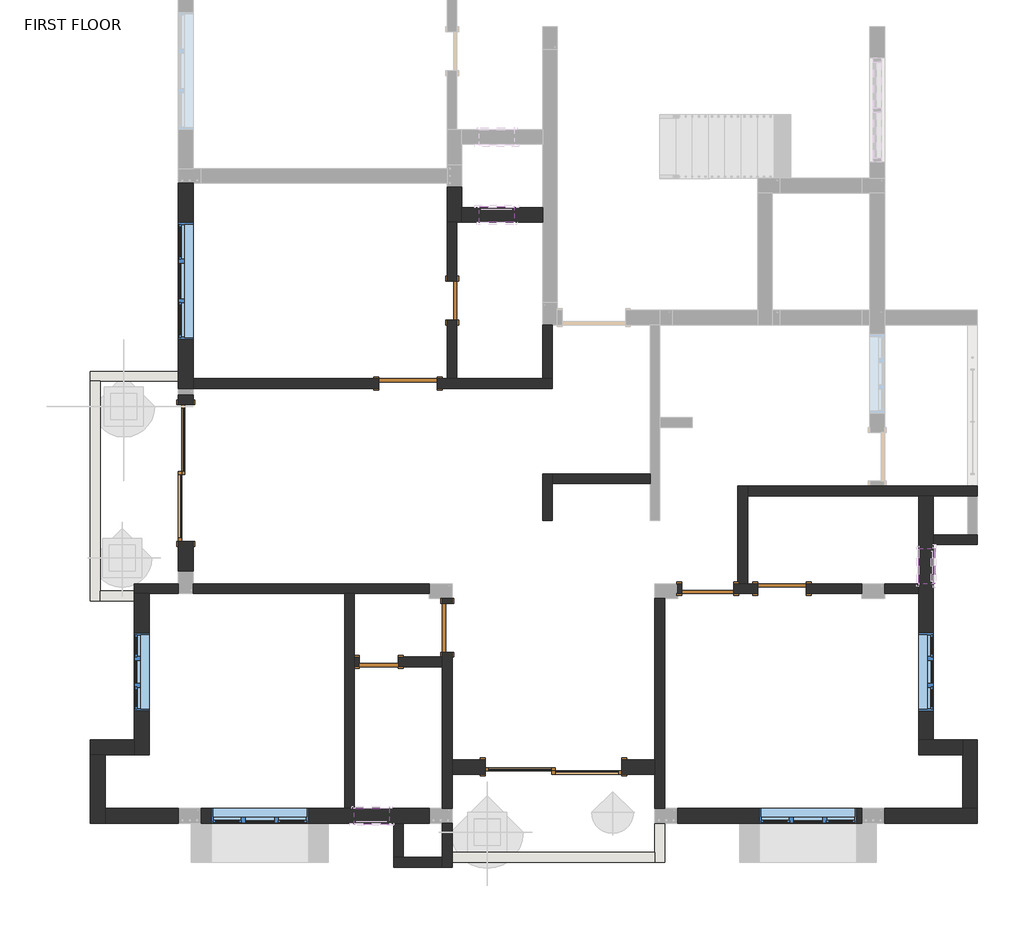
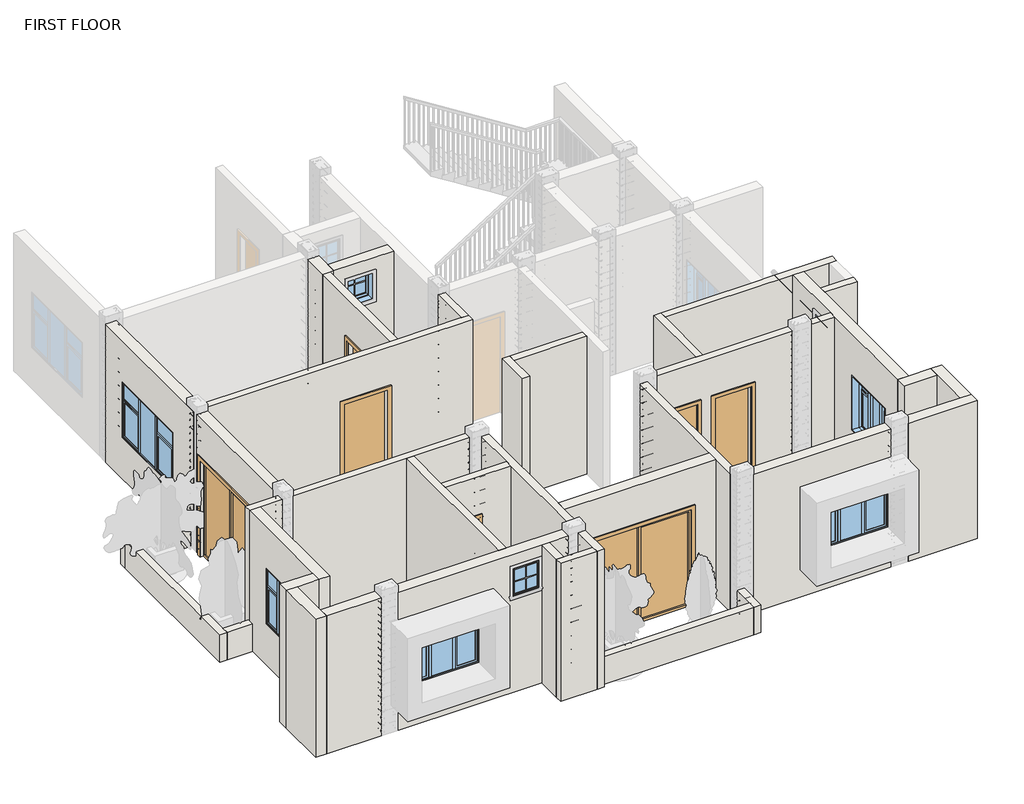
# One storey, part 1 of 10: 39 walls, 8 doors, 8 windows.
"""IFC4 building model written with IfcOpenShell, lengths in millimetres."""

from ifc_helpers import new_model, si_unit, frame, origin, place, context, project, spatial, polyline, outline, extrude, faceted_brep, transform, mapped, element, save
from components import door_double_sliding_7_x7_ddbaaa7c, door_e2b13fe9, door_377e7377, single_flush_2_x7_9ea4ff49, single_flush_3_x7_16372e1c, window_casement_triple_side_transom_4_x4_2_fd24aed3, window_casement_triple_side_transom_5_x4_f59ddf0b, window_casement_triple_side_transom_6_x4_596ba82f, window_6ec6991e

model = new_model("IFC4")

# Units and contexts
model_context = context("Model", 3, world=origin())
ifc_project = project(units=[si_unit("LENGTHUNIT", "METRE", prefix="MILLI")], contexts=[model_context])

# Site, building, storey
site = spatial("IfcSite", under=ifc_project)
building = spatial("IfcBuilding", under=site)
storey = spatial("IfcBuildingStorey", under=building, Name="FIRST FLOOR", Elevation=3200.4)

# Doors
placement = place(None, origin())
door_double_sliding_7_x7_shape = door_double_sliding_7_x7_ddbaaa7c(model_context)
element("IfcDoor", 1, ObjectType="Door-Double-Sliding : 7'X7'", at=placement, inside=storey, context=model_context, shape_type="MappedRepresentation", body=[
    mapped(door_double_sliding_7_x7_shape, transform((-403.8333787, -9045.640066, 3200.4), x_axis=(-1.0, 0.0, 0.0), y_axis=(0.0, -1.0, 0.0), z_axis=(0.0, 0.0, 1.0))),
])
element("IfcDoor", 2, ObjectType="Door-Double-Sliding : 7'X7'", at=placement, inside=storey, context=model_context, shape_type="MappedRepresentation", body=[
    mapped(door_double_sliding_7_x7_shape, transform((-6010.8833787, -4587.940066, 3200.4), x_axis=(0.0, 1.0, 0.0), y_axis=(-1.0, 0.0, 0.0), z_axis=(0.0, 0.0, 1.0))),
])
door_shape = door_e2b13fe9(model_context)
element("IfcDoor", 3, ObjectType="Single-Flush : 2'6\"X7'", at=placement, inside=storey, context=model_context, shape_type="MappedRepresentation", body=[
    mapped(door_shape, transform((-2061.1833787, -7000.940066, 3200.4), x_axis=(0.0, -1.0, 0.0), y_axis=(1.0, 0.0, 0.0), z_axis=(0.0, 0.0, 1.0))),
])
element("IfcDoor", 4, ObjectType="Single-Flush : 2'6\"X7'", at=placement, inside=storey, context=model_context, shape_type="MappedRepresentation", body=[
    mapped(door_shape, transform((3158.5166213, -6391.340066, 3200.4), x_axis=(-1.0, 0.0, 0.0), y_axis=(0.0, -1.0, 0.0), z_axis=(0.0, 0.0, 1.0))),
])
door_2_shape = door_377e7377(model_context)
element("IfcDoor", 5, ObjectType="Single-Flush : 2'8\"X7'", at=placement, inside=storey, context=model_context, shape_type="MappedRepresentation", body=[
    mapped(door_2_shape, transform((2002.8166213, -6391.340066, 3200.4), x_axis=(-1.0, 0.0, 0.0), y_axis=(0.0, -1.0, 0.0), z_axis=(0.0, 0.0, 1.0))),
])
single_flush_2_x7_shape = single_flush_2_x7_9ea4ff49(model_context)
element("IfcDoor", 6, ObjectType="Single-Flush : 2'X7'", at=placement, inside=storey, context=model_context, shape_type="MappedRepresentation", body=[
    mapped(single_flush_2_x7_shape, transform((-3127.9833787, -7534.340066, 3200.4), x_axis=(-1.0, 0.0, 0.0), y_axis=(0.0, -1.0, 0.0), z_axis=(0.0, 0.0, 1.0))),
])
element("IfcDoor", 7, ObjectType="Single-Flush : 2'X7'", at=placement, inside=storey, context=model_context, shape_type="MappedRepresentation", body=[
    mapped(single_flush_2_x7_shape, transform((-1984.9833787, -1895.540066, 3200.4), x_axis=(0.0, -1.0, 0.0), y_axis=(1.0, 0.0, 0.0), z_axis=(0.0, 0.0, 1.0))),
])
single_flush_3_x7_shape = single_flush_3_x7_16372e1c(model_context)
element("IfcDoor", 8, ObjectType="Single-Flush : 3'X7'", at=placement, inside=storey, context=model_context, shape_type="MappedRepresentation", body=[
    mapped(single_flush_3_x7_shape, transform((-2670.7833787, -3190.940066, 3200.4), x_axis=(1.0, 0.0, 0.0), y_axis=(0.0, 1.0, 0.0), z_axis=(0.0, 0.0, 1.0))),
])

# Walls
element("IfcWall", 9, ObjectType="6\"", at=placement, inside=storey, context=model_context, shape_type="SweptSolid", body=[
    extrude(outline(polyline([(-2200.340066, 5334.0), (-2200.340066, 3200.4), (-3114.740066, 3200.4), (-3114.740066, 6248.4), (-676.340066, 6248.4), (-676.340066, 3200.4), (-1590.740066, 3200.4), (-1590.740066, 5334.0), (-2200.340066, 5334.0)])), frame((-2061.1833787, 0.0, 0.0), z_axis=(1.0, 0.0, 0.0), x_axis=(0.0, 1.0, 0.0)), (0.0, 0.0, 1.0), 152.4),
])
element("IfcWall", 10, ObjectType="6\"", at=placement, inside=storey, context=model_context, shape_type="Brep", body=[
    faceted_brep([(-2213.5833787, -3267.140066, 5334.0), (-2213.5833787, -3267.140066, 3200.4), (-422.8833787, -3267.140066, 3200.4), (-422.8833787, -3267.140066, 6248.4), (-6023.5833787, -3267.140066, 6248.4), (-6023.5833787, -3267.140066, 3810.0), (-6023.5833787, -3267.140066, 3200.4), (-3127.9833787, -3267.140066, 3200.4), (-3127.9833787, -3267.140066, 5334.0), (-422.8833787, -3114.740066, 3200.4), (-575.2833787, -3114.740066, 3200.4), (-1908.7833787, -3114.740066, 3200.4), (-2061.1833787, -3114.740066, 3200.4), (-2213.5833787, -3114.740066, 3200.4), (-2213.5833787, -3114.740066, 5334.0), (-3127.9833787, -3114.740066, 5334.0), (-3127.9833787, -3114.740066, 3200.4), (-6023.5833787, -3114.740066, 3200.4), (-6023.5833787, -3114.740066, 6248.4), (-2061.1833787, -3114.740066, 6248.4), (-1908.7833787, -3114.740066, 6248.4), (-575.2833787, -3114.740066, 6248.4), (-422.8833787, -3114.740066, 6248.4), (-6023.5833787, -3152.840066, 3200.4)], [[[0, 1, 2, 3, 4, 5, 6, 7, 8]], [[9, 10, 11, 12, 13, 14, 15, 16, 17, 18, 19, 20, 21, 22]], [[7, 6, 23, 17, 16]], [[2, 1, 13, 12, 11, 10, 9]], [[4, 3, 22, 21, 20, 19, 18]], [[3, 2, 9, 22]], [[14, 13, 1, 0]], [[15, 14, 0, 8]], [[16, 15, 8, 7]], [[6, 5, 4, 18, 17, 23]]]),
])
element("IfcWall", 11, ObjectType="6\"", at=placement, inside=storey, context=model_context, shape_type="SweptSolid", body=[
    extrude(outline(polyline([(-422.8833787, -2276.540066), (-422.8833787, -3114.740066), (-575.2833787, -3114.740066), (-575.2833787, -2276.540066), (-422.8833787, -2276.540066)])), frame((0.0, 0.0, 3200.4), z_axis=(0.0, 0.0, 1.0), x_axis=(1.0, 0.0, 0.0)), (0.0, 0.0, 1.0), 3048.0),
])
element("IfcWall", 12, ObjectType="6\"", at=placement, inside=storey, context=model_context, shape_type="Brep", body=[
    faceted_brep([(-6937.9833787, -6467.540066, 6248.4), (-6937.9833787, -6467.540066, 3200.4), (-6709.3833787, -6467.540066, 3200.4), (-6252.1833787, -6467.540066, 3200.4), (-6252.1833787, -6467.540066, 6248.4), (-6709.3833787, -6467.540066, 6248.4), (-6937.9833787, -6315.140066, 3200.4), (-6937.9833787, -6315.140066, 6248.4), (-6252.1833787, -6315.140066, 6248.4), (-6252.1833787, -6315.140066, 3200.4), (-6937.9833787, -6429.440066, 3200.4)], [[[0, 1, 2, 3, 4, 5]], [[6, 7, 8, 9]], [[3, 2, 1, 10, 6, 9]], [[4, 3, 9, 8]], [[0, 5, 4, 8, 7]], [[0, 7, 6, 10, 1]]]),
])
element("IfcWall", 13, ObjectType="6\"", at=placement, inside=storey, context=model_context, shape_type="Brep", body=[
    faceted_brep([(-6023.5833787, -6467.540066, 3200.4), (-3661.3833787, -6467.540066, 3200.4), (-3508.9833787, -6467.540066, 3200.4), (-2340.5833787, -6467.540066, 3200.4), (-2340.5833787, -6467.540066, 6248.4), (-3508.9833787, -6467.540066, 6248.4), (-3661.3833787, -6467.540066, 6248.4), (-6023.5833787, -6467.540066, 6248.4), (-6023.5833787, -6315.140066, 3200.4), (-6023.5833787, -6315.140066, 6248.4), (-2340.5833787, -6315.140066, 6248.4), (-2340.5833787, -6315.140066, 3200.4)], [[[0, 1, 2, 3, 4, 5, 6, 7]], [[8, 9, 10, 11]], [[3, 2, 1, 0, 8, 11]], [[4, 3, 11, 10]], [[7, 6, 5, 4, 10, 9]], [[0, 7, 9, 8]]]),
])
element("IfcWall", 14, ObjectType="6\"", at=placement, inside=storey, context=model_context, shape_type="Brep", body=[
    faceted_brep([(-3508.9833787, -9820.340066, 3200.4), (-3508.9833787, -7610.540066, 3200.4), (-3508.9833787, -7458.140066, 3200.4), (-3508.9833787, -6467.540066, 3200.4), (-3508.9833787, -6467.540066, 6248.4), (-3508.9833787, -7458.140066, 6248.4), (-3508.9833787, -7610.540066, 6248.4), (-3508.9833787, -9820.340066, 6248.4), (-3508.9833787, -9820.340066, 5943.6), (-3508.9833787, -9820.340066, 5334.0), (-3661.3833787, -9820.340066, 3200.4), (-3661.3833787, -9820.340066, 6248.4), (-3661.3833787, -6467.540066, 6248.4), (-3661.3833787, -6467.540066, 3200.4)], [[[0, 1, 2, 3, 4, 5, 6, 7, 8, 9]], [[10, 11, 12, 13]], [[3, 2, 1, 0, 10, 13]], [[7, 6, 5, 4, 12, 11]], [[0, 9, 8, 7, 11, 10]], [[4, 3, 13, 12]]]),
])
element("IfcWall", 15, ObjectType="6\"", at=placement, inside=storey, context=model_context, shape_type="Brep", body=[
    faceted_brep([(-1984.9833787, -9820.340066, 3200.4), (-1984.9833787, -9286.940066, 3200.4), (-1984.9833787, -9058.340066, 3200.4), (-1984.9833787, -7381.940066, 3200.4), (-1984.9833787, -7381.940066, 5334.0), (-1984.9833787, -6619.940066, 5334.0), (-1984.9833787, -6619.940066, 3200.4), (-1984.9833787, -6543.740066, 3200.4), (-1984.9833787, -6543.740066, 6248.4), (-1984.9833787, -9058.340066, 6248.4), (-1984.9833787, -9286.940066, 6248.4), (-1984.9833787, -9820.340066, 6248.4), (-2137.3833787, -7381.940066, 5334.0), (-2137.3833787, -7381.940066, 3200.4), (-2137.3833787, -7458.140066, 3200.4), (-2137.3833787, -7610.540066, 3200.4), (-2137.3833787, -9820.340066, 3200.4), (-2137.3833787, -9820.340066, 6248.4), (-2137.3833787, -7610.540066, 6248.4), (-2137.3833787, -7458.140066, 6248.4), (-2137.3833787, -6543.740066, 6248.4), (-2137.3833787, -6543.740066, 3200.4), (-2137.3833787, -6619.940066, 3200.4), (-2137.3833787, -6619.940066, 5334.0)], [[[0, 1, 2, 3, 4, 5, 6, 7, 8, 9, 10, 11]], [[12, 13, 14, 15, 16, 17, 18, 19, 20, 21, 22, 23]], [[22, 21, 7, 6]], [[16, 15, 14, 13, 3, 2, 1, 0]], [[8, 7, 21, 20]], [[11, 10, 9, 8, 20, 19, 18, 17]], [[0, 11, 17, 16]], [[4, 3, 13, 12]], [[5, 4, 12, 23]], [[6, 5, 23, 22]]]),
])
element("IfcWall", 16, ObjectType="6\"", at=placement, inside=storey, context=model_context, shape_type="SweptSolid", body=[
    extrude(outline(polyline([(3200.4, -3508.9833787), (3200.4, -3432.7833787), (5334.0, -3432.7833787), (5334.0, -2823.1833787), (3200.4, -2823.1833787), (3200.4, -2137.3833787), (6248.4, -2137.3833787), (6248.4, -3508.9833787), (3200.4, -3508.9833787)])), frame((0.0, -7610.540066, 0.0), z_axis=(0.0, 1.0, 0.0), x_axis=(0.0, 0.0, 1.0)), (0.0, 0.0, 1.0), 152.4),
])
element("IfcWall", 17, ObjectType="6\"", at=placement, inside=storey, context=model_context, shape_type="Brep", body=[
    faceted_brep([(-2137.3833787, -10048.940066, 3200.4), (-2137.3833787, -10582.340066, 3200.4), (-2137.3833787, -10734.740066, 3200.4), (-2137.3833787, -10734.740066, 6248.4), (-2137.3833787, -10582.340066, 6248.4), (-2137.3833787, -10048.940066, 6248.4), (-1984.9833787, -10048.940066, 3200.4), (-1984.9833787, -10048.940066, 6248.4), (-1984.9833787, -10734.740066, 6248.4), (-1984.9833787, -10734.740066, 3200.4), (-1984.9833787, -10658.540066, 3200.4), (-1984.9833787, -10506.140066, 3200.4)], [[[0, 1, 2, 3, 4, 5]], [[6, 7, 8, 9, 10, 11]], [[2, 1, 0, 6, 11, 10, 9]], [[5, 4, 3, 8, 7]], [[0, 5, 7, 6]], [[2, 9, 8, 3]]]),
])
element("IfcWall", 18, ObjectType="6\"", at=placement, inside=storey, context=model_context, shape_type="Brep", body=[
    faceted_brep([(-2137.3833787, -10582.340066, 6248.4), (-2137.3833787, -10582.340066, 3200.4), (-2746.3100526, -10582.340066, 3200.4), (-2898.7100526, -10582.340066, 3200.4), (-2898.7100526, -10582.340066, 6248.4), (-2746.3100526, -10582.340066, 6248.4), (-2137.3833787, -10734.740066, 3200.4), (-2137.3833787, -10734.740066, 6248.4), (-2898.7100526, -10734.740066, 6248.4), (-2898.7100526, -10734.740066, 3200.4)], [[[0, 1, 2, 3, 4, 5]], [[6, 7, 8, 9]], [[3, 2, 1, 6, 9]], [[0, 5, 4, 8, 7]], [[4, 3, 9, 8]], [[0, 7, 6, 1]]]),
])
element("IfcWall", 19, ObjectType="6\"", at=placement, inside=storey, context=model_context, shape_type="SweptSolid", body=[
    extrude(outline(polyline([(-2746.3100526, -10048.940066), (-2746.3100526, -10582.340066), (-2898.7100526, -10582.340066), (-2898.7100526, -10048.940066), (-2746.3100526, -10048.940066)])), frame((0.0, 0.0, 3200.4), z_axis=(0.0, 0.0, 1.0), x_axis=(1.0, 0.0, 0.0)), (0.0, 0.0, 1.0), 3048.0),
])
element("IfcWall", 20, ObjectType="6\"", at=placement, inside=storey, context=model_context, shape_type="Brep", body=[
    faceted_brep([(1177.3166213, -10048.940066, 3200.4), (1177.3166213, -10506.140066, 3200.4), (1177.3166213, -10658.540066, 3200.4), (1177.3166213, -10658.540066, 3810.0), (1177.3166213, -10506.140066, 3810.0), (1177.3166213, -10048.940066, 3810.0), (1329.7166213, -10048.940066, 3200.4), (1329.7166213, -10048.940066, 3810.0), (1329.7166213, -10658.540066, 3810.0), (1329.7166213, -10658.540066, 3200.4)], [[[0, 1, 2, 3, 4, 5]], [[6, 7, 8, 9]], [[2, 1, 0, 6, 9]], [[5, 4, 3, 8, 7]], [[0, 5, 7, 6]], [[3, 2, 9, 8]]]),
])
element("IfcWall", 21, ObjectType="6\"", at=placement, inside=storey, context=model_context, shape_type="SweptSolid", body=[
    extrude(outline(polyline([(-1984.9833787, -10506.140066), (1177.3166213, -10506.140066), (1177.3166213, -10658.540066), (-1984.9833787, -10658.540066), (-1984.9833787, -10506.140066)])), frame((0.0, 0.0, 3200.4), z_axis=(0.0, 0.0, 1.0), x_axis=(1.0, 0.0, 0.0)), (0.0, 0.0, 1.0), 609.6),
])
element("IfcWall", 22, ObjectType="6\"", at=placement, inside=storey, context=model_context, shape_type="Brep", body=[
    faceted_brep([(1329.7166213, -9820.340066, 3200.4), (1329.7166213, -6543.740066, 3200.4), (1329.7166213, -6543.740066, 6248.4), (1329.7166213, -9820.340066, 6248.4), (1177.3166213, -9820.340066, 3200.4), (1177.3166213, -9820.340066, 6248.4), (1177.3166213, -9286.940066, 6248.4), (1177.3166213, -9058.340066, 6248.4), (1177.3166213, -6543.740066, 6248.4), (1177.3166213, -6543.740066, 3200.4), (1177.3166213, -9058.340066, 3200.4), (1177.3166213, -9286.940066, 3200.4)], [[[0, 1, 2, 3]], [[4, 5, 6, 7, 8, 9, 10, 11]], [[1, 0, 4, 11, 10, 9]], [[2, 1, 9, 8]], [[3, 2, 8, 7, 6, 5]], [[0, 3, 5, 4]]]),
])
element("IfcWall", 23, ObjectType="6\"", at=placement, inside=storey, context=model_context, shape_type="Brep", body=[
    faceted_brep([(2409.2166213, -6467.540066, 3200.4), (2777.5166213, -6467.540066, 3200.4), (2777.5166213, -6467.540066, 5334.0), (3539.5166213, -6467.540066, 5334.0), (3539.5166213, -6467.540066, 3200.4), (4403.1166213, -6467.540066, 3200.4), (4403.1166213, -6467.540066, 6248.4), (1532.9166213, -6467.540066, 6248.4), (1532.9166213, -6467.540066, 3200.4), (1596.4166213, -6467.540066, 3200.4), (1596.4166213, -6467.540066, 5334.0), (2409.2166213, -6467.540066, 5334.0), (2777.5166213, -6315.140066, 5334.0), (2777.5166213, -6315.140066, 3200.4), (2625.1166213, -6315.140066, 3200.4), (2472.7166213, -6315.140066, 3200.4), (2409.2166213, -6315.140066, 3200.4), (2409.2166213, -6315.140066, 5334.0), (1596.4166213, -6315.140066, 5334.0), (1596.4166213, -6315.140066, 3200.4), (1532.9166213, -6315.140066, 3200.4), (1532.9166213, -6315.140066, 6248.4), (2472.7166213, -6315.140066, 6248.4), (2625.1166213, -6315.140066, 6248.4), (4403.1166213, -6315.140066, 6248.4), (4403.1166213, -6315.140066, 3200.4), (3539.5166213, -6315.140066, 3200.4), (3539.5166213, -6315.140066, 5334.0)], [[[0, 1, 2, 3, 4, 5, 6, 7, 8, 9, 10, 11]], [[12, 13, 14, 15, 16, 17, 18, 19, 20, 21, 22, 23, 24, 25, 26, 27]], [[20, 19, 9, 8]], [[26, 25, 5, 4]], [[16, 15, 14, 13, 1, 0]], [[6, 5, 25, 24]], [[7, 6, 24, 23, 22, 21]], [[8, 7, 21, 20]], [[10, 9, 19, 18]], [[11, 10, 18, 17]], [[0, 11, 17, 16]], [[2, 1, 13, 12]], [[3, 2, 12, 27]], [[4, 3, 27, 26]]]),
])
element("IfcWall", 24, ObjectType="6\"", at=placement, inside=storey, context=model_context, shape_type="SweptSolid", body=[
    extrude(outline(polyline([(5292.1166213, -6467.540066), (4758.7166213, -6467.540066), (4758.7166213, -6315.140066), (5292.1166213, -6315.140066), (5292.1166213, -6467.540066)])), frame((0.0, 0.0, 3200.4), z_axis=(0.0, 0.0, 1.0), x_axis=(1.0, 0.0, 0.0)), (0.0, 0.0, 1.0), 3048.0),
])
element("IfcWall", 25, ObjectType="6\"", at=placement, inside=storey, context=model_context, shape_type="Brep", body=[
    faceted_brep([(2625.1166213, -6315.140066, 3200.4), (2625.1166213, -4943.540066, 3200.4), (2625.1166213, -4791.140066, 3200.4), (2625.1166213, -4791.140066, 6248.4), (2625.1166213, -4943.540066, 6248.4), (2625.1166213, -6315.140066, 6248.4), (2472.7166213, -6315.140066, 3200.4), (2472.7166213, -6315.140066, 6248.4), (2472.7166213, -4791.140066, 6248.4), (2472.7166213, -4791.140066, 3200.4)], [[[0, 1, 2, 3, 4, 5]], [[6, 7, 8, 9]], [[2, 1, 0, 6, 9]], [[5, 4, 3, 8, 7]], [[0, 5, 7, 6]], [[3, 2, 9, 8]]]),
])
element("IfcWall", 26, ObjectType="6\"", at=placement, inside=storey, context=model_context, shape_type="Brep", body=[
    faceted_brep([(2625.1166213, -4943.540066, 3200.4), (5292.1166213, -4943.540066, 3200.4), (5520.7166213, -4943.540066, 3200.4), (6054.1166213, -4943.540066, 3200.4), (6054.1166213, -4943.540066, 3810.0), (6206.5166213, -4943.540066, 3810.0), (6206.5166213, -4943.540066, 6248.4), (6054.1166213, -4943.540066, 6248.4), (5520.7166213, -4943.540066, 6248.4), (5292.1166213, -4943.540066, 6248.4), (2625.1166213, -4943.540066, 6248.4), (2625.1166213, -4791.140066, 3200.4), (2625.1166213, -4791.140066, 6248.4), (4530.1166213, -4791.140066, 6248.4), (4758.7166213, -4791.140066, 6248.4), (6206.5166213, -4791.140066, 6248.4), (6206.5166213, -4791.140066, 3810.0), (6054.1166213, -4791.140066, 3810.0), (6054.1166213, -4791.140066, 3200.4), (4758.7166213, -4791.140066, 3200.4), (4530.1166213, -4791.140066, 3200.4)], [[[0, 1, 2, 3, 4, 5, 6, 7, 8, 9, 10]], [[11, 12, 13, 14, 15, 16, 17, 18, 19, 20]], [[3, 2, 1, 0, 11, 20, 19, 18]], [[10, 9, 8, 7, 6, 15, 14, 13, 12]], [[0, 10, 12, 11]], [[16, 5, 4, 17]], [[4, 3, 18, 17]], [[6, 5, 16, 15]]]),
])
element("IfcWall", 27, ObjectType="6\"", at=placement, inside=storey, context=model_context, shape_type="Brep", body=[
    faceted_brep([(-422.8833787, -5324.540066, 3200.4), (-422.8833787, -4753.040066, 3200.4), (-422.8833787, -4600.640066, 3200.4), (-422.8833787, -4600.640066, 6248.4), (-422.8833787, -4753.040066, 6248.4), (-422.8833787, -5324.540066, 6248.4), (-575.2833787, -5324.540066, 3200.4), (-575.2833787, -5324.540066, 6248.4), (-575.2833787, -4600.640066, 6248.4), (-575.2833787, -4600.640066, 3200.4)], [[[0, 1, 2, 3, 4, 5]], [[6, 7, 8, 9]], [[2, 1, 0, 6, 9]], [[5, 4, 3, 8, 7]], [[0, 5, 7, 6]], [[3, 2, 9, 8]]]),
])
element("IfcWall", 28, ObjectType="6\"", at=placement, inside=storey, context=model_context, shape_type="SweptSolid", body=[
    extrude(outline(polyline([(1101.1166213, -4753.040066), (-422.8833787, -4753.040066), (-422.8833787, -4600.640066), (1101.1166213, -4600.640066), (1101.1166213, -4753.040066)])), frame((0.0, 0.0, 3200.4), z_axis=(0.0, 0.0, 1.0), x_axis=(1.0, 0.0, 0.0)), (0.0, 0.0, 1.0), 3048.0),
])
element("IfcWall", 29, ObjectType="6\"", at=placement, inside=storey, context=model_context, shape_type="Brep", body=[
    faceted_brep([(6206.5166213, -5552.4667399, 3200.4), (6054.1166213, -5552.4667399, 3200.4), (5520.7166213, -5552.4667399, 3200.4), (5520.7166213, -5552.4667399, 6248.4), (6054.1166213, -5552.4667399, 6248.4), (6206.5166213, -5552.4667399, 6248.4), (6206.5166213, -5704.8667399, 3200.4), (6206.5166213, -5704.8667399, 6248.4), (5520.7166213, -5704.8667399, 6248.4), (5520.7166213, -5704.8667399, 3200.4)], [[[0, 1, 2, 3, 4, 5]], [[6, 7, 8, 9]], [[2, 1, 0, 6, 9]], [[5, 4, 3, 8, 7]], [[3, 2, 9, 8]], [[0, 5, 7, 6]]]),
])
element("IfcWall", 30, ObjectType="6\"", at=placement, inside=storey, context=model_context, shape_type="Brep", body=[
    faceted_brep([(-6252.1833787, -3000.440066, 3200.4), (-7623.7833787, -3000.440066, 3200.4), (-7623.7833787, -3000.440066, 3810.0), (-6252.1833787, -3000.440066, 3810.0), (-6252.1833787, -3152.840066, 3200.4), (-6252.1833787, -3152.840066, 3810.0), (-7471.3833787, -3152.840066, 3810.0), (-7623.7833787, -3152.840066, 3810.0), (-7623.7833787, -3152.840066, 3200.4), (-7471.3833787, -3152.840066, 3200.4)], [[[0, 1, 2, 3]], [[4, 5, 6, 7, 8, 9]], [[1, 0, 4, 9, 8]], [[3, 2, 7, 6, 5]], [[0, 3, 5, 4]], [[2, 1, 8, 7]]]),
])
element("IfcWall", 31, ObjectType="6\"", at=placement, inside=storey, context=model_context, shape_type="Brep", body=[
    faceted_brep([(-7623.7833787, -3152.840066, 3200.4), (-7623.7833787, -6581.840066, 3200.4), (-7623.7833787, -6581.840066, 3810.0), (-7623.7833787, -3152.840066, 3810.0), (-7471.3833787, -3152.840066, 3200.4), (-7471.3833787, -3152.840066, 3810.0), (-7471.3833787, -6429.440066, 3810.0), (-7471.3833787, -6581.840066, 3810.0), (-7471.3833787, -6581.840066, 3200.4), (-7471.3833787, -6429.440066, 3200.4)], [[[0, 1, 2, 3]], [[4, 5, 6, 7, 8, 9]], [[1, 0, 4, 9, 8]], [[3, 2, 7, 6, 5]], [[0, 3, 5, 4]], [[2, 1, 8, 7]]]),
])
element("IfcWall", 32, ObjectType="6\"", at=placement, inside=storey, context=model_context, shape_type="Brep", body=[
    faceted_brep([(-7471.3833787, -6581.840066, 3200.4), (-6937.9833787, -6581.840066, 3200.4), (-6937.9833787, -6581.840066, 3810.0), (-7471.3833787, -6581.840066, 3810.0), (-7471.3833787, -6429.440066, 3200.4), (-7471.3833787, -6429.440066, 3810.0), (-6937.9833787, -6429.440066, 3810.0), (-6937.9833787, -6429.440066, 3200.4), (-6937.9833787, -6467.540066, 3200.4)], [[[0, 1, 2, 3]], [[4, 5, 6, 7]], [[1, 0, 4, 7, 8]], [[3, 2, 6, 5]], [[0, 3, 5, 4]], [[2, 1, 8, 7, 6]]]),
])
element("IfcWall", 33, ObjectType="9\"", at=placement, inside=storey, context=model_context, shape_type="Brep", body=[
    faceted_brep([(-6252.1833787, -66.740066, 3200.4), (-6252.1833787, -3000.440066, 3200.4), (-6252.1833787, -3152.840066, 3200.4), (-6252.1833787, -3152.840066, 3810.0), (-6252.1833787, -3267.140066, 3810.0), (-6252.1833787, -3267.140066, 6248.4), (-6252.1833787, -66.740066, 6248.4), (-6252.1833787, -676.340066, 5334.0), (-6252.1833787, -2505.140066, 5334.0), (-6252.1833787, -2505.140066, 4114.8), (-6252.1833787, -676.340066, 4114.8), (-6023.5833787, -66.740066, 3200.4), (-6023.5833787, -66.740066, 6248.4), (-6023.5833787, -3114.740066, 6248.4), (-6023.5833787, -3267.140066, 6248.4), (-6023.5833787, -3267.140066, 3810.0), (-6023.5833787, -3152.840066, 3810.0), (-6023.5833787, -3152.840066, 3200.4), (-6023.5833787, -3114.740066, 3200.4), (-6023.5833787, -676.340066, 5334.0), (-6023.5833787, -676.340066, 4114.8), (-6023.5833787, -2505.140066, 4114.8), (-6023.5833787, -2505.140066, 5334.0)], [[[0, 1, 2, 3, 4, 5, 6], [7, 8, 9, 10]], [[11, 12, 13, 14, 15, 16, 17, 18], [19, 20, 21, 22]], [[2, 1, 0, 11, 18, 17]], [[6, 5, 14, 13, 12]], [[0, 6, 12, 11]], [[20, 19, 7, 10]], [[21, 20, 10, 9]], [[22, 21, 9, 8]], [[19, 22, 8, 7]], [[15, 4, 3, 16]], [[3, 2, 17, 16]], [[5, 4, 15, 14]]]),
])
element("IfcWall", 34, ObjectType="9\"", at=placement, inside=storey, context=model_context, shape_type="SweptSolid", body=[
    extrude(outline(polyline([(-3368.740066, 3200.4), (-3521.140066, 3200.4), (-3521.140066, 5334.0), (-5654.740066, 5334.0), (-5654.740066, 3200.4), (-6111.940066, 3200.4), (-6111.940066, 6248.4), (-3368.740066, 6248.4), (-3368.740066, 3200.4)])), frame((-6252.1833787, 0.0, 0.0), z_axis=(1.0, 0.0, 0.0), x_axis=(0.0, 1.0, 0.0)), (0.0, 0.0, 1.0), 228.6),
])
element("IfcWall", 35, ObjectType="9\"", at=placement, inside=storey, context=model_context, shape_type="Brep", body=[
    faceted_brep([(-6937.9833787, -6467.540066, 3200.4), (-6937.9833787, -6581.840066, 3200.4), (-6937.9833787, -8753.540066, 3200.4), (-6937.9833787, -8982.140066, 3200.4), (-6937.9833787, -8982.140066, 6248.4), (-6937.9833787, -8753.540066, 6248.4), (-6937.9833787, -6467.540066, 6248.4), (-6937.9833787, -7079.7633095, 5334.0), (-6937.9833787, -8298.9633095, 5334.0), (-6937.9833787, -8298.9633095, 4114.8), (-6937.9833787, -7079.7633095, 4114.8), (-6709.3833787, -6467.540066, 3200.4), (-6709.3833787, -6467.540066, 6248.4), (-6709.3833787, -8982.140066, 6248.4), (-6709.3833787, -8982.140066, 3200.4), (-6709.3833787, -7079.7633095, 5334.0), (-6709.3833787, -7079.7633095, 4114.8), (-6709.3833787, -8298.9633095, 4114.8), (-6709.3833787, -8298.9633095, 5334.0)], [[[0, 1, 2, 3, 4, 5, 6], [7, 8, 9, 10]], [[11, 12, 13, 14], [15, 16, 17, 18]], [[3, 2, 1, 0, 11, 14]], [[6, 5, 4, 13, 12]], [[4, 3, 14, 13]], [[0, 6, 12, 11]], [[16, 15, 7, 10]], [[17, 16, 10, 9]], [[18, 17, 9, 8]], [[15, 18, 8, 7]]]),
])
element("IfcWall", 36, ObjectType="9\"", at=placement, inside=storey, context=model_context, shape_type="Brep", body=[
    faceted_brep([(-6937.9833787, -8753.540066, 3200.4), (-7623.7833787, -8753.540066, 3200.4), (-7623.7833787, -8753.540066, 6248.4), (-6937.9833787, -8753.540066, 6248.4), (-6937.9833787, -8982.140066, 3200.4), (-6937.9833787, -8982.140066, 6248.4), (-7395.1833787, -8982.140066, 6248.4), (-7623.7833787, -8982.140066, 6248.4), (-7623.7833787, -8982.140066, 3200.4), (-7395.1833787, -8982.140066, 3200.4)], [[[0, 1, 2, 3]], [[4, 5, 6, 7, 8, 9]], [[1, 0, 4, 9, 8]], [[3, 2, 7, 6, 5]], [[0, 3, 5, 4]], [[2, 1, 8, 7]]]),
])
element("IfcWall", 37, ObjectType="9\"", at=placement, inside=storey, context=model_context, shape_type="Brep", body=[
    faceted_brep([(-7623.7833787, -8982.140066, 3200.4), (-7623.7833787, -10048.940066, 3200.4), (-7623.7833787, -10048.940066, 6248.4), (-7623.7833787, -8982.140066, 6248.4), (-7395.1833787, -8982.140066, 3200.4), (-7395.1833787, -8982.140066, 6248.4), (-7395.1833787, -9820.340066, 6248.4), (-7395.1833787, -10048.940066, 6248.4), (-7395.1833787, -10048.940066, 3200.4), (-7395.1833787, -9820.340066, 3200.4)], [[[0, 1, 2, 3]], [[4, 5, 6, 7, 8, 9]], [[1, 0, 4, 9, 8]], [[3, 2, 7, 6, 5]], [[0, 3, 5, 4]], [[2, 1, 8, 7]]]),
])
element("IfcWall", 38, ObjectType="9\"", at=placement, inside=storey, context=model_context, shape_type="Brep", body=[
    faceted_brep([(-7395.1833787, -10048.940066, 3200.4), (-6252.1833787, -10048.940066, 3200.4), (-6252.1833787, -10048.940066, 6248.4), (-7395.1833787, -10048.940066, 6248.4), (-7395.1833787, -10048.940066, 3429.0), (-7395.1833787, -10048.940066, 3276.6), (-7395.1833787, -9820.340066, 3200.4), (-7395.1833787, -9820.340066, 6248.4), (-6252.1833787, -9820.340066, 6248.4), (-6252.1833787, -9820.340066, 3200.4)], [[[0, 1, 2, 3, 4, 5]], [[6, 7, 8, 9]], [[1, 0, 6, 9]], [[2, 1, 9, 8]], [[3, 2, 8, 7]], [[0, 5, 4, 3, 7, 6]]]),
])
element("IfcWall", 39, ObjectType="9\"", at=placement, inside=storey, context=model_context, shape_type="Brep", body=[
    faceted_brep([(-5896.5833787, -10048.940066, 3200.4), (-2898.7100526, -10048.940066, 3200.4), (-2746.3100526, -10048.940066, 3200.4), (-2340.5833787, -10048.940066, 3200.4), (-2340.5833787, -10048.940066, 6248.4), (-2746.3100526, -10048.940066, 6248.4), (-2898.7100526, -10048.940066, 6248.4), (-5896.5833787, -10048.940066, 6248.4), (-5744.1833787, -10048.940066, 5334.0), (-4220.1833787, -10048.940066, 5334.0), (-4220.1833787, -10048.940066, 4114.8), (-5744.1833787, -10048.940066, 4114.8), (-3508.9833787, -10048.940066, 5943.6), (-2962.8833787, -10048.940066, 5943.6), (-2962.8833787, -10048.940066, 5334.0), (-3508.9833787, -10048.940066, 5334.0), (-5896.5833787, -9820.340066, 3200.4), (-5896.5833787, -9820.340066, 6248.4), (-3661.3833787, -9820.340066, 6248.4), (-3508.9833787, -9820.340066, 6248.4), (-2340.5833787, -9820.340066, 6248.4), (-2340.5833787, -9820.340066, 3200.4), (-3508.9833787, -9820.340066, 3200.4), (-3661.3833787, -9820.340066, 3200.4), (-5744.1833787, -9820.340066, 5334.0), (-5744.1833787, -9820.340066, 4114.8), (-4220.1833787, -9820.340066, 4114.8), (-4220.1833787, -9820.340066, 5334.0), (-3508.9833787, -9820.340066, 5943.6), (-3508.9833787, -9820.340066, 5334.0), (-2962.8833787, -9820.340066, 5334.0), (-2962.8833787, -9820.340066, 5943.6)], [[[0, 1, 2, 3, 4, 5, 6, 7], [8, 9, 10, 11], [12, 13, 14, 15]], [[16, 17, 18, 19, 20, 21, 22, 23], [24, 25, 26, 27], [28, 29, 30, 31]], [[3, 2, 1, 0, 16, 23, 22, 21]], [[4, 3, 21, 20]], [[7, 6, 5, 4, 20, 19, 18, 17]], [[0, 7, 17, 16]], [[25, 24, 8, 11]], [[26, 25, 11, 10]], [[27, 26, 10, 9]], [[24, 27, 9, 8]], [[29, 28, 12, 15]], [[30, 29, 15, 14]], [[31, 30, 14, 13]], [[28, 31, 13, 12]]]),
])
element("IfcWall", 40, ObjectType="9\"", at=placement, inside=storey, context=model_context, shape_type="SweptSolid", body=[
    extrude(outline(polyline([(3200.4, -1984.9833787), (3200.4, -1470.6333787), (5334.0, -1470.6333787), (5334.0, 662.9666213), (3200.4, 662.9666213), (3200.4, 1177.3166213), (6248.4, 1177.3166213), (6248.4, -1984.9833787), (3200.4, -1984.9833787)])), frame((0.0, -9286.940066, 0.0), z_axis=(0.0, 1.0, 0.0), x_axis=(0.0, 0.0, 1.0)), (0.0, 0.0, 1.0), 228.6),
])
element("IfcWall", 41, ObjectType="9\"", at=placement, inside=storey, context=model_context, shape_type="SweptSolid", body=[
    extrude(outline(polyline([(3200.4, 1532.9166213), (3200.4, 4403.1166213), (6248.4, 4403.1166213), (6248.4, 1532.9166213), (3200.4, 1532.9166213)]), holes=[polyline([(5334.0, 2802.9166213), (5334.0, 4326.9166213), (4114.8, 4326.9166213), (4114.8, 2802.9166213), (5334.0, 2802.9166213)])]), frame((0.0, -10048.940066, 0.0), z_axis=(0.0, 1.0, 0.0), x_axis=(0.0, 0.0, 1.0)), (0.0, 0.0, 1.0), 228.6),
])
element("IfcWall", 42, ObjectType="9\"", at=placement, inside=storey, context=model_context, shape_type="Brep", body=[
    faceted_brep([(4758.7166213, -10048.940066, 3200.4), (6206.5166213, -10048.940066, 3200.4), (6206.5166213, -10048.940066, 6248.4), (4758.7166213, -10048.940066, 6248.4), (4758.7166213, -9820.340066, 3200.4), (4758.7166213, -9820.340066, 6248.4), (5977.9166213, -9820.340066, 6248.4), (6206.5166213, -9820.340066, 6248.4), (6206.5166213, -9820.340066, 3200.4), (5977.9166213, -9820.340066, 3200.4)], [[[0, 1, 2, 3]], [[4, 5, 6, 7, 8, 9]], [[1, 0, 4, 9, 8]], [[3, 2, 7, 6, 5]], [[0, 3, 5, 4]], [[2, 1, 8, 7]]]),
])
element("IfcWall", 43, ObjectType="9\"", at=placement, inside=storey, context=model_context, shape_type="Brep", body=[
    faceted_brep([(6206.5166213, -9820.340066, 3200.4), (6206.5166213, -8753.540066, 3200.4), (6206.5166213, -8753.540066, 6248.4), (6206.5166213, -9820.340066, 6248.4), (5977.9166213, -9820.340066, 3200.4), (5977.9166213, -9820.340066, 6248.4), (5977.9166213, -8982.140066, 6248.4), (5977.9166213, -8753.540066, 6248.4), (5977.9166213, -8753.540066, 3200.4), (5977.9166213, -8982.140066, 3200.4)], [[[0, 1, 2, 3]], [[4, 5, 6, 7, 8, 9]], [[1, 0, 4, 9, 8]], [[3, 2, 7, 6, 5]], [[0, 3, 5, 4]], [[2, 1, 8, 7]]]),
])
element("IfcWall", 44, ObjectType="9\"", at=placement, inside=storey, context=model_context, shape_type="Brep", body=[
    faceted_brep([(5977.9166213, -8753.540066, 3200.4), (5520.7166213, -8753.540066, 3200.4), (5292.1166213, -8753.540066, 3200.4), (5292.1166213, -8753.540066, 6248.4), (5520.7166213, -8753.540066, 6248.4), (5977.9166213, -8753.540066, 6248.4), (5977.9166213, -8982.140066, 3200.4), (5977.9166213, -8982.140066, 6248.4), (5292.1166213, -8982.140066, 6248.4), (5292.1166213, -8982.140066, 3200.4)], [[[0, 1, 2, 3, 4, 5]], [[6, 7, 8, 9]], [[2, 1, 0, 6, 9]], [[5, 4, 3, 8, 7]], [[0, 5, 7, 6]], [[3, 2, 9, 8]]]),
])
element("IfcWall", 45, ObjectType="9\"", at=placement, inside=storey, context=model_context, shape_type="Brep", body=[
    faceted_brep([(5520.7166213, -8753.540066, 3200.4), (5520.7166213, -5704.8667399, 3200.4), (5520.7166213, -5552.4667399, 3200.4), (5520.7166213, -4943.540066, 3200.4), (5520.7166213, -4943.540066, 6248.4), (5520.7166213, -5552.4667399, 6248.4), (5520.7166213, -5704.8667399, 6248.4), (5520.7166213, -8753.540066, 6248.4), (5520.7166213, -8298.9633095, 5334.0), (5520.7166213, -7079.7633095, 5334.0), (5520.7166213, -7079.7633095, 4114.8), (5520.7166213, -8298.9633095, 4114.8), (5520.7166213, -6313.7934138, 5943.6), (5520.7166213, -5767.6934138, 5943.6), (5520.7166213, -5767.6934138, 5334.0), (5520.7166213, -6313.7934138, 5334.0), (5292.1166213, -8753.540066, 3200.4), (5292.1166213, -8753.540066, 6248.4), (5292.1166213, -6467.540066, 6248.4), (5292.1166213, -6315.140066, 6248.4), (5292.1166213, -4943.540066, 6248.4), (5292.1166213, -4943.540066, 3200.4), (5292.1166213, -6315.140066, 3200.4), (5292.1166213, -6467.540066, 3200.4), (5292.1166213, -8298.9633095, 5334.0), (5292.1166213, -8298.9633095, 4114.8), (5292.1166213, -7079.7633095, 4114.8), (5292.1166213, -7079.7633095, 5334.0), (5292.1166213, -6313.7934138, 5943.6), (5292.1166213, -6313.7934138, 5334.0), (5292.1166213, -5767.6934138, 5334.0), (5292.1166213, -5767.6934138, 5943.6)], [[[0, 1, 2, 3, 4, 5, 6, 7], [8, 9, 10, 11], [12, 13, 14, 15]], [[16, 17, 18, 19, 20, 21, 22, 23], [24, 25, 26, 27], [28, 29, 30, 31]], [[3, 2, 1, 0, 16, 23, 22, 21]], [[7, 6, 5, 4, 20, 19, 18, 17]], [[0, 7, 17, 16]], [[4, 3, 21, 20]], [[25, 24, 8, 11]], [[26, 25, 11, 10]], [[27, 26, 10, 9]], [[24, 27, 9, 8]], [[29, 28, 12, 15]], [[30, 29, 15, 14]], [[31, 30, 14, 13]], [[28, 31, 13, 12]]]),
])
element("IfcWall", 46, ObjectType="9\"", at=placement, inside=storey, context=model_context, shape_type="SweptSolid", body=[
    extrude(outline(polyline([(3200.4, -575.2833787), (6248.4, -575.2833787), (6248.4, -1832.5833787), (3200.4, -1832.5833787), (3200.4, -575.2833787)]), holes=[polyline([(5943.6, -1013.4333787), (5334.0, -1013.4333787), (5334.0, -1559.5333787), (5943.6, -1559.5333787), (5943.6, -1013.4333787)])]), frame((0.0, -676.340066, 0.0), z_axis=(0.0, 1.0, 0.0), x_axis=(0.0, 0.0, 1.0)), (0.0, 0.0, 1.0), 228.6),
])
element("IfcWall", 47, ObjectType="9\"", at=placement, inside=storey, context=model_context, shape_type="Brep", body=[
    faceted_brep([(-1832.5833787, -676.340066, 3200.4), (-1832.5833787, -447.740066, 3200.4), (-1832.5833787, -130.240066, 3200.4), (-1832.5833787, -130.240066, 6248.4), (-1832.5833787, -447.740066, 6248.4), (-1832.5833787, -676.340066, 6248.4), (-2061.1833787, -676.340066, 3200.4), (-2061.1833787, -676.340066, 6248.4), (-2061.1833787, -130.240066, 6248.4), (-2061.1833787, -130.240066, 3200.4), (-1908.7833787, -676.340066, 3200.4), (-1908.7833787, -676.340066, 6248.4)], [[[0, 1, 2, 3, 4, 5]], [[6, 7, 8, 9]], [[2, 1, 0, 10, 6, 9]], [[3, 2, 9, 8]], [[5, 4, 3, 8, 7, 11]], [[0, 5, 11, 7, 6, 10]]]),
])

# Windows
window_casement_triple_side_transom_4_x4_2_shape = window_casement_triple_side_transom_4_x4_2_fd24aed3(model_context)
element("IfcWindow", 48, ObjectType="Window-Casement-Triple-Side-Transom : 4'X4' 2", at=placement, inside=storey, context=model_context, shape_type="MappedRepresentation", body=[
    mapped(window_casement_triple_side_transom_4_x4_2_shape, transform((-6823.6833787, -7689.3633095, 3200.4), x_axis=(0.0, 1.0, 0.0), y_axis=(-1.0, 0.0, 0.0), z_axis=(0.0, 0.0, 1.0))),
])
element("IfcWindow", 49, ObjectType="Window-Casement-Triple-Side-Transom : 4'X4' 2", at=placement, inside=storey, context=model_context, shape_type="MappedRepresentation", body=[
    mapped(window_casement_triple_side_transom_4_x4_2_shape, transform((5406.4166213, -7689.3633095, 3200.4), x_axis=(0.0, -1.0, 0.0), y_axis=(1.0, 0.0, 0.0), z_axis=(0.0, 0.0, 1.0))),
])
window_casement_triple_side_transom_5_x4_shape = window_casement_triple_side_transom_5_x4_f59ddf0b(model_context)
element("IfcWindow", 50, ObjectType="Window-Casement-Triple-Side-Transom : 5'X4'", at=placement, inside=storey, context=model_context, shape_type="MappedRepresentation", body=[
    mapped(window_casement_triple_side_transom_5_x4_shape, transform((-4982.1833787, -9934.640066, 3200.4), x_axis=(-1.0, 0.0, 0.0), y_axis=(0.0, -1.0, 0.0), z_axis=(0.0, 0.0, 1.0))),
])
element("IfcWindow", 51, ObjectType="Window-Casement-Triple-Side-Transom : 5'X4'", at=placement, inside=storey, context=model_context, shape_type="MappedRepresentation", body=[
    mapped(window_casement_triple_side_transom_5_x4_shape, transform((3564.9166213, -9934.640066, 3200.4), x_axis=(-1.0, 0.0, 0.0), y_axis=(0.0, -1.0, 0.0), z_axis=(0.0, 0.0, 1.0))),
])
window_casement_triple_side_transom_6_x4_shape = window_casement_triple_side_transom_6_x4_596ba82f(model_context)
element("IfcWindow", 52, ObjectType="Window-Casement-Triple-Side-Transom : 6'X4'", at=placement, inside=storey, context=model_context, shape_type="MappedRepresentation", body=[
    mapped(window_casement_triple_side_transom_6_x4_shape, transform((-6137.8833787, -1590.740066, 3200.4), x_axis=(0.0, 1.0, 0.0), y_axis=(-1.0, 0.0, 0.0), z_axis=(0.0, 0.0, 1.0))),
])
window_shape = window_6ec6991e(model_context)
element("IfcWindow", 53, ObjectType="Window-Fixed : 1'9.5\"X2'", at=placement, inside=storey, context=model_context, shape_type="MappedRepresentation", body=[
    mapped(window_shape, transform((-3235.9333787, -9934.640066, 3200.4), x_axis=(-1.0, 0.0, 0.0), y_axis=(0.0, -1.0, 0.0), z_axis=(0.0, 0.0, 1.0))),
])
element("IfcWindow", 54, ObjectType="Window-Fixed : 1'9.5\"X2'", at=placement, inside=storey, context=model_context, shape_type="MappedRepresentation", body=[
    mapped(window_shape, transform((5406.4166213, -6040.7434138, 3200.4), x_axis=(0.0, -1.0, 0.0), y_axis=(1.0, 0.0, 0.0), z_axis=(0.0, 0.0, 1.0))),
])
element("IfcWindow", 55, ObjectType="Window-Fixed : 1'9.5\"X2'", at=placement, inside=storey, context=model_context, shape_type="MappedRepresentation", body=[
    mapped(window_shape, transform((-1286.4833787, -562.040066, 3200.4), x_axis=(1.0, 0.0, 0.0), y_axis=(0.0, 1.0, 0.0), z_axis=(0.0, 0.0, 1.0))),
])

save(model, "model.ifc")

# Revit data of these elements
# Type "Door-Double-Sliding : 7'X7'"
#   Type Mark = "14"
#   Construction Type Id = "opn-d45"
#   Assembly Code = "C1020"
#   Analytic Construction = "Wood frame, double glass door "
#   Thickness = 0' - 2"
#   Thermal Resistance (R) = 1.8150 (h·ft²·°F)/BTU
#   Heat Transfer Coefficient (U) = 0.5510 BTU/(h·ft²·°F)
#   Height = 7' - 0"
#   Rail Width = 0' - 2"
#   Stiles = 0' - 2"
#   Trim Projection Ext = 0' - 1"
#   Trim Projection Int = 0' - 1"
#   Trim Width = 0' - 3"
#   Width = 7' - 0"
#   Define Thermal Properties by = 1
#   Glazing = Glass
#   Panel Material = Wood - Birch - Solid Stained Light Low Gloss
#   Trim Material = Paint - Sienna
#   Visual Light Transmittance = 0
#   Solar Heat Gain Coefficient = 0
#   Function = (empty or 0)
#   Wall Closure = (empty or 0)
# Type "Single-Flush : 2'6\"X7'"
#   Type Mark = "10"
#   Construction Type Id = "MDOOR"
#   Assembly Code = "C1020"
#   Analytic Construction = "Metal"
#   Thickness = 0' - 2"
#   Heat Transfer Coefficient (U) = 0.651978 BTU/(h·ft²·°F)
#   Height = 7' - 0"
#   Trim Projection Ext = 0' - 1"
#   Trim Projection Int = 0' - 1"
#   Trim Width = 0' - 3"
#   Width = 2' - 6"
#   Define Thermal Properties by = 1
#   Door Material = Door - Panel
#   Frame Material = Door - Frame
#   Visual Light Transmittance = 0
#   Solar Heat Gain Coefficient = 0
#   Function = (empty or 0)
#   Wall Closure = (empty or 0)
# Type "Single-Flush : 2'8\"X7'"
#   Type Mark = "9"
#   Construction Type Id = "MDOOR"
#   Assembly Code = "C1020"
#   Analytic Construction = "Metal"
#   Thickness = 0' - 2"
#   Heat Transfer Coefficient (U) = 0.651978 BTU/(h·ft²·°F)
#   Height = 7' - 0"
#   Trim Projection Ext = 0' - 1"
#   Trim Projection Int = 0' - 1"
#   Trim Width = 0' - 3"
#   Width = 2' - 8"
#   Define Thermal Properties by = 1
#   Door Material = Door - Panel
#   Frame Material = Door - Frame
#   Visual Light Transmittance = 0
#   Solar Heat Gain Coefficient = 0
#   Function = (empty or 0)
#   Wall Closure = (empty or 0)
# Type "Single-Flush : 2'X7'"
#   Type Mark = "12"
#   Construction Type Id = "MDOOR"
#   Assembly Code = "C1020"
#   Analytic Construction = "Metal"
#   Thickness = 0' - 2"
#   Heat Transfer Coefficient (U) = 0.651978 BTU/(h·ft²·°F)
#   Height = 7' - 0"
#   Trim Projection Ext = 0' - 1"
#   Trim Projection Int = 0' - 1"
#   Trim Width = 0' - 3"
#   Width = 2' - 0"
#   Define Thermal Properties by = 1
#   Door Material = Door - Panel
#   Frame Material = Door - Frame
#   Visual Light Transmittance = 0
#   Solar Heat Gain Coefficient = 0
#   Function = (empty or 0)
#   Wall Closure = (empty or 0)
# Type "Single-Flush : 3'X7'"
#   Type Mark = "8"
#   Construction Type Id = "MDOOR"
#   Assembly Code = "C1020"
#   Analytic Construction = "Metal"
#   Thickness = 0' - 2"
#   Heat Transfer Coefficient (U) = 0.651978 BTU/(h·ft²·°F)
#   Height = 7' - 0"
#   Trim Projection Ext = 0' - 1"
#   Trim Projection Int = 0' - 1"
#   Trim Width = 0' - 3"
#   Width = 3' - 0"
#   Define Thermal Properties by = 1
#   Door Material = Door - Panel
#   Frame Material = Door - Frame
#   Visual Light Transmittance = 0
#   Solar Heat Gain Coefficient = 0
#   Function = (empty or 0)
#   Wall Closure = (empty or 0)
# Type "6\""
#   Assembly Code = "B2010"
#   Layers, outside or top first: 0' - 6" "6\" wall" (function 1)
# Type "9\""
#   Assembly Code = "B2010"
#   Layers, outside or top first: 0' - 9" "charcoal grey" (function 1)
# Type "Window-Casement-Triple-Side-Transom : 4'X4' 2"
#   Type Mark = "26"
#   Fire Rating = "0.5h"
#   Assembly Code = "B2020100"
#   Analytic Construction = "Double glazing - domestic"
#   Window Width = 1' - 4"
#   Window Inset [instance default] = 0' - 0 5/8"
#   Wall Thickness [instance default] = 0' - 6"
#   Visual Light Transmittance = 0.81
#   Transom Height Ratio = 0.3
#   Thermal Resistance (R) = 1.8146 (h·ft²·°F)/BTU
#   Solar Heat Gain Coefficient = 0.76
#   Rough Width = 4' - 0 1/2"
#   Rough Height = 4' - 0 1/2"
#   Open Window Height = 2' - 9.6"
#   Heat Transfer Coefficient (U) = 0.5511 BTU/(h·ft²·°F)
#   Height = 4' - 0"
#   Transom Height = 1' - 2.4"
#   Frame Gap 3 [instance default] = 0' - 1 83/128"
#   Frame Gap 2 [instance default] = 0' - 0 5/8"
#   Frame Gap 1 = 0' - 1 51/128"
#   Default Sill Height = 3' - 0"
#   Width = 4' - 0"
#   Frame Material = Metal - Aluminum
#   Glass Panel Material = Glass
#   Wall Closure = (empty or 0)
# Type "Window-Casement-Triple-Side-Transom : 5'X4'"
#   Type Mark = "24"
#   Fire Rating = "0.5h"
#   Assembly Code = "B2020100"
#   Analytic Construction = "Double glazing - domestic"
#   Window Width = 1' - 8"
#   Window Inset [instance default] = 0' - 0 5/8"
#   Wall Thickness [instance default] = 0' - 6"
#   Visual Light Transmittance = 0.81
#   Transom Height Ratio = 0.3
#   Thermal Resistance (R) = 1.8146 (h·ft²·°F)/BTU
#   Solar Heat Gain Coefficient = 0.76
#   Rough Width = 5' - 0 1/2"
#   Rough Height = 4' - 0 1/2"
#   Open Window Height = 2' - 9.6"
#   Heat Transfer Coefficient (U) = 0.5511 BTU/(h·ft²·°F)
#   Height = 4' - 0"
#   Transom Height = 1' - 2.4"
#   Frame Gap 3 [instance default] = 0' - 1 83/128"
#   Frame Gap 2 [instance default] = 0' - 0 5/8"
#   Frame Gap 1 = 0' - 1 51/128"
#   Default Sill Height = 3' - 0"
#   Width = 5' - 0"
#   Frame Material = Metal - Aluminum
#   Glass Panel Material = Glass
#   Wall Closure = (empty or 0)
# Type "Window-Casement-Triple-Side-Transom : 6'X4'"
#   Type Mark = "23"
#   Fire Rating = "0.5h"
#   Assembly Code = "B2020100"
#   Analytic Construction = "Double glazing - domestic"
#   Window Width = 2' - 0"
#   Window Inset [instance default] = 0' - 0 5/8"
#   Wall Thickness [instance default] = 0' - 6"
#   Visual Light Transmittance = 0.81
#   Transom Height Ratio = 0.3
#   Thermal Resistance (R) = 1.8146 (h·ft²·°F)/BTU
#   Solar Heat Gain Coefficient = 0.76
#   Rough Width = 6' - 0 1/2"
#   Rough Height = 4' - 0 1/2"
#   Open Window Height = 2' - 9.6"
#   Heat Transfer Coefficient (U) = 0.5511 BTU/(h·ft²·°F)
#   Height = 4' - 0"
#   Transom Height = 1' - 2.4"
#   Frame Gap 3 [instance default] = 0' - 1 83/128"
#   Frame Gap 2 [instance default] = 0' - 0 5/8"
#   Frame Gap 1 = 0' - 1 51/128"
#   Default Sill Height = 3' - 0"
#   Width = 6' - 0"
#   Frame Material = Metal - Aluminum
#   Glass Panel Material = Glass
#   Wall Closure = (empty or 0)
# Type "Window-Fixed : 1'9.5\"X2'"
#   Type Mark = "29"
#   Fire Rating = "0.5h"
#   Assembly Code = "B2020100"
#   Analytic Construction = "Double glazing - domestic"
#   Window Inset [instance default] = 0' - 0"
#   Wall Thickness [instance default] = 0' - 6"
#   Visual Light Transmittance = 0.81
#   Thermal Resistance (R) = 1.8146 (h·ft²·°F)/BTU
#   Solar Heat Gain Coefficient = 0.76
#   Rough Width = 1' - 10"
#   Rough Height = 2' - 0 1/2"
#   Interior Wall Closure [instance default] = 0' - 2 1/4"
#   Height = 2' - 0"
#   Heat Transfer Coefficient (U) = 0.5511 BTU/(h·ft²·°F)
#   Frame Extension [instance default] = 0' - 0 1/4"
#   Exterior Wall Closure [instance default] = 0' - 1 1/4"
#   Extension Jamb [instance default] = 0' - 2 1/4"
#   Default Sill Height = 7' - 0"
#   Width = 1' - 9 1/2"
#   Muntin Visibility = yes
#   Interior Trim Visibility [instance default] = yes
#   Exterior Trim Visibility [instance default] = yes
#   Extension Jamb Visibility [instance default] = yes
#   Muntin Pattern = Muntin Pattern_2x2 : Muntin Pattern_2x2
#   Interior Trim Material = Wood - Stained
#   Interior Trim = Trim-Window-Interior-Flat : Picture Frame
#   Interior Frame Material = Wood - Stained
#   Glass Panel Material = Glass
#   Exterior Trim Material = Clad - White
#   Exterior Trim = Trim-Window-Exterior-Flat : with Sill
#   Exterior Frame Material = Clad - White
#   Wall Closure = (empty or 0)
# Elements 1, 2 (IfcDoor, "Door-Double-Sliding : 7'X7'")
#   Phase Created = New Construction
#   Materials on its faces: "Paint - Sienna", "Wood - Birch - Solid Stained Light Low Gloss", "Glass"
# Elements 3, 4 (IfcDoor, "Single-Flush : 2'6\"X7'")
#   Phase Created = New Construction
#   Materials on its faces: "Door - Frame", "Door - Panel"
# Element 5 (IfcDoor, "Single-Flush : 2'8\"X7'")
#   Phase Created = New Construction
#   Materials on its faces: "Door - Frame", "Door - Panel"
# Elements 6, 7 (IfcDoor, "Single-Flush : 2'X7'")
#   Phase Created = New Construction
#   Materials on its faces: "Door - Frame", "Door - Panel"
# Element 8 (IfcDoor, "Single-Flush : 3'X7'")
#   Phase Created = New Construction
#   Materials on its faces: "Door - Frame", "Door - Panel"
# Elements 9, 10, 11, 13, 14, 16, 23, 24, 25, 26, 27, 28, 29 (IfcWall, "6\"")
#   Top Offset = -0' - 6"
#   Base Offset = 0' - 0"
#   wall height = 10' - 0"
#   Phase Created = New Construction
#   Base Constraint = FIRST FLOOR
#   Top Constraint = SECOND FLOOR
#   Materials on its faces: "6\" wall"
# Elements 12, 15, 17, 18, 19, 22 (IfcWall, "6\"")
#   Top Offset = -0' - 6"
#   Base Offset = 0' - 0"
#   wall height = 10' - 0"
#   Phase Created = New Construction
#   Base Constraint = FIRST FLOOR
#   Top Constraint = SECOND FLOOR
#   Materials on its faces: "6\" wall", "charcoal grey"
# Elements 20, 21 (IfcWall, "6\"")
#   Top Offset = 0' - 0"
#   Base Offset = 0' - 0"
#   Unconnected Height = 2' - 0"
#   wall height = 2' - 0"
#   Phase Created = New Construction
#   Base Constraint = FIRST FLOOR
#   Materials on its faces: "6\" wall", "wood 1", "Asphalt, Pavement, Light Grey"
# Elements 30, 31, 32 (IfcWall, "6\"")
#   Top Offset = 0' - 0"
#   Base Offset = 0' - 0"
#   Unconnected Height = 2' - 0"
#   wall height = 2' - 0"
#   Phase Created = New Construction
#   Base Constraint = FIRST FLOOR
#   Materials on its faces: "6\" wall"
# Element 33 (IfcWall, "9\"")
#   Top Offset = -0' - 6"
#   Base Offset = 0' - 0"
#   wall height = 10' - 0"
#   Phase Created = New Construction
#   Base Constraint = FIRST FLOOR
#   Top Constraint = SECOND FLOOR
#   Materials on its faces: "charcoal grey", "6\" wall", "Asphalt, Pavement, Light Grey"
# Elements 34, 35, 36, 37, 38, 39, 41, 42, 43, 44, 45, 46, 47 (IfcWall, "9\"")
#   Top Offset = -0' - 6"
#   Base Offset = 0' - 0"
#   wall height = 10' - 0"
#   Phase Created = New Construction
#   Base Constraint = FIRST FLOOR
#   Top Constraint = SECOND FLOOR
#   Materials on its faces: "charcoal grey"
# Element 40 (IfcWall, "9\"")
#   Top Offset = -0' - 6"
#   Base Offset = 0' - 0"
#   wall height = 10' - 0"
#   Phase Created = New Construction
#   Base Constraint = FIRST FLOOR
#   Top Constraint = SECOND FLOOR
#   Materials on its faces: "charcoal grey", "Asphalt, Pavement, Light Grey"
# Element 48 (IfcWindow, "Window-Casement-Triple-Side-Transom : 4'X4' 2")
#   Mark = "24"
#   Window Inset = 0' - 0 5/8"
#   Frame Gap 3 = 0' - 1 83/128"
#   Frame Gap 2 = 0' - 0 5/8"
#   Phase Created = New Construction
#   Materials on its faces: "Metal - Aluminum", "Glass"
# Element 49 (IfcWindow, "Window-Casement-Triple-Side-Transom : 4'X4' 2")
#   Mark = "25"
#   Window Inset = 0' - 0 5/8"
#   Frame Gap 3 = 0' - 1 83/128"
#   Frame Gap 2 = 0' - 0 5/8"
#   Phase Created = New Construction
#   Materials on its faces: "Metal - Aluminum", "Glass"
# Element 50 (IfcWindow, "Window-Casement-Triple-Side-Transom : 5'X4'")
#   Mark = "29"
#   Window Inset = 0' - 0 5/8"
#   Frame Gap 3 = 0' - 1 83/128"
#   Frame Gap 2 = 0' - 0 5/8"
#   Phase Created = New Construction
#   Materials on its faces: "Metal - Aluminum", "Glass"
# Element 51 (IfcWindow, "Window-Casement-Triple-Side-Transom : 5'X4'")
#   Mark = "30"
#   Window Inset = 0' - 0 5/8"
#   Frame Gap 3 = 0' - 1 83/128"
#   Frame Gap 2 = 0' - 0 5/8"
#   Phase Created = New Construction
#   Materials on its faces: "Metal - Aluminum", "Glass"
# Element 52 (IfcWindow, "Window-Casement-Triple-Side-Transom : 6'X4'")
#   Mark = "21"
#   Window Inset = 0' - 0 5/8"
#   Frame Gap 3 = 0' - 1 83/128"
#   Frame Gap 2 = 0' - 0 5/8"
#   Phase Created = New Construction
#   Materials on its faces: "Metal - Aluminum", "Glass"
# Element 53 (IfcWindow, "Window-Fixed : 1'9.5\"X2'")
#   Mark = "32"
#   Window Inset = 0' - 0"
#   Interior Wall Closure = 0' - 2 1/4"
#   Frame Extension = 0' - 0 1/4"
#   Exterior Wall Closure = 0' - 1 1/4"
#   Interior Trim Visibility = yes
#   Exterior Trim Visibility = yes
#   Phase Created = New Construction
#   Materials on its faces: "Wood - Stained", "Glass", "Clad - White"
# Element 54 (IfcWindow, "Window-Fixed : 1'9.5\"X2'")
#   Mark = "33"
#   Window Inset = 0' - 0"
#   Interior Wall Closure = 0' - 2 1/4"
#   Frame Extension = 0' - 0 1/4"
#   Exterior Wall Closure = 0' - 1 1/4"
#   Interior Trim Visibility = yes
#   Exterior Trim Visibility = yes
#   Phase Created = New Construction
#   Materials on its faces: "Wood - Stained", "Glass", "Clad - White"
# Element 55 (IfcWindow, "Window-Fixed : 1'9.5\"X2'")
#   Mark = "36"
#   Window Inset = 0' - 0"
#   Interior Wall Closure = 0' - 2 1/4"
#   Frame Extension = 0' - 0 1/4"
#   Exterior Wall Closure = 0' - 1 1/4"
#   Interior Trim Visibility = yes
#   Exterior Trim Visibility = yes
#   Phase Created = New Construction
#   Materials on its faces: "Wood - Stained", "Glass", "Clad - White"
# Materials
#   "Glass": class "Glass", colour RGB 0 128 192, transparency 0.75, Description = "Soda Lime Glass", Cost = 0
#   "Wood - Birch - Solid Stained Light Low Gloss": class "Wood", colour RGB 210 159 95, transparency 0, Cost = 0
#   "Paint - Sienna": colour RGB 118 70 51, transparency 0, Cost = 0
#   "Door - Panel": class "Wood", colour RGB 210 159 95, transparency 0, Cost = 0
#   "Door - Frame": colour RGB 118 70 51, transparency 0, Cost = 0
#   "6\" wall": class "Generic", colour RGB 245 239 227, transparency 0, Cost = 0
#   "charcoal grey": class "Generic", colour RGB 54 69 79, transparency 0, Cost = 0
#   "Metal - Aluminum": class "Metal", colour RGB 247 247 247, transparency 0
#   "Wood - Stained": class "Wood", colour RGB 224 178 126, transparency 0, Cost = 0
#   "Clad - White": class "Wood", colour RGB 242 242 238, transparency 0, Cost = 0
#   "wood 1": class "Generic", colour RGB 119 107 117, transparency 0, Cost = 0
#   "Asphalt, Pavement, Light Grey": class "Generic", colour RGB 120 120 120, transparency 0, Description = "Asphalt or tarmac paving", Cost = 0
